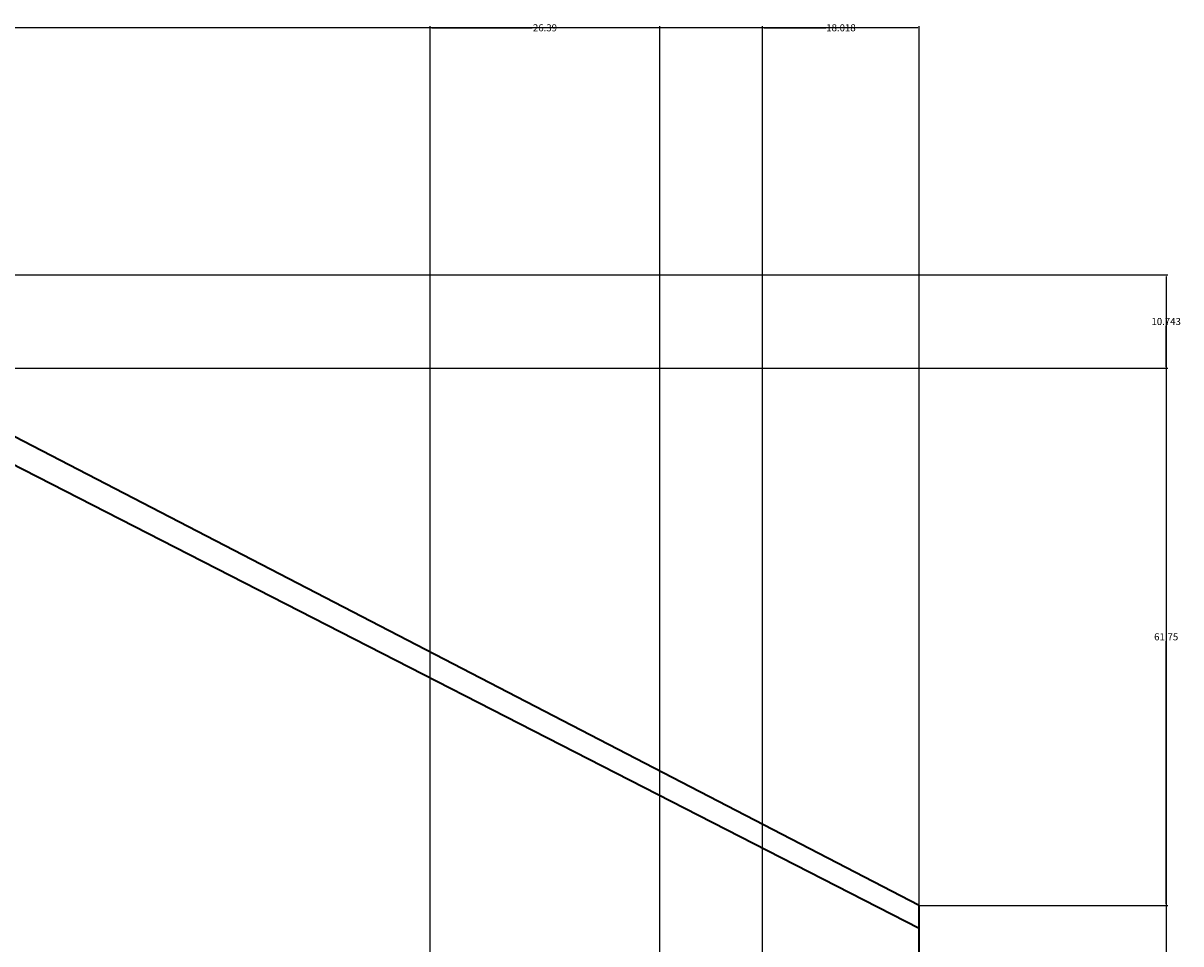
# Model space of a CAD drawing. Units: inches. Extents: x 69 to 650, y -16 to 573.
# Tile 26 of 26: x 516 to 650, y 467 to 573. Entities that reach past the tile are written whole.
import ezdxf

# ---------------------------------------------------------------- set-up
doc = ezdxf.new("R2010")
doc.units = ezdxf.units.IN
doc.header["$MEASUREMENT"] = 0
for name, color, linetype, lineweight in [('A-ANNO-DIMS', 2, 'Continuous', 18), ('A-ROOF', 7, 'Continuous', 35), ('A-WALL', 7, 'Continuous', 35)]:
    doc.layers.add(name, color=color, linetype=linetype, lineweight=lineweight)
doc.styles.get("Standard").update_dxf_attribs({"font": 'arial.ttf'})
doc.dimstyles.get("Standard").update_dxf_attribs({"dimtxt": 0.8125, "dimasz": 0.18, "dimexe": 0.18, "dimexo": 0.0625, "dimgap": 0.09, "dimtad": 0, "dimtih": 1, "dimtoh": 1, "dimdec": 4, "dimzin": 0, "dimdsep": 46, "dimlunit": 4, "dimtxsty": 'Standard', "dimcen": 0.09, "dimadec": 0, "dimazin": 0, "dimtfac": 1, "dimtdec": 4, "dimtofl": 0, "dimtmove": 0, "dimatfit": 3, "dimfxl": 1, "dimtolj": 1, "dimtzin": 0, "dimarcsym": 0})

# ---------------------------------------------------------------- blocks, each defined once
blk = doc.blocks.new('*D19')
at = {"layer": 'A-ANNO-DIMS', "color": 0, "lineweight": -2, "transparency": 16777216}
for p, q in [((99.56, 471.72), (99.56, 572.74)), ((619.56, 87.99), (619.56, 572.74)), ((99.74, 572.56), (358.57, 572.56)), ((619.38, 572.56), (360.54, 572.56))]:
    blk.add_line(p, q, dxfattribs=at)
at = {"layer": 'A-ANNO-DIMS', "color": 0, "transparency": 16777216}
for points in [[(99.74, 572.59), (99.74, 572.53), (99.56, 572.56)], [(619.38, 572.59), (619.38, 572.53), (619.56, 572.56)]]:
    blk.add_solid(points, dxfattribs=at)
at = {"layer": 'Defpoints', "color": 0, "transparency": 16777216}
for p in [(619.56, 572.56), (99.56, 471.66), (619.56, 87.93)]:
    blk.add_point(p, dxfattribs=at)
at = {"layer": 'A-ANNO-DIMS', "color": 0, "transparency": 16777216, "insert": (359.56, 572.56), "char_height": 0.812, "attachment_point": 5}
blk.add_mtext('\\A1;520', dxfattribs=at)
blk = doc.blocks.new('*D20')
at = {"layer": 'A-ANNO-DIMS', "color": 0, "lineweight": -2, "transparency": 16777216}
for p, q in [((504.24, 544.16), (648.14, 544.16)), ((647.96, 543.98), (647.96, 304.55)), ((647.96, 64.11), (647.96, 303.54)), ((619.62, 63.93), (648.14, 63.93))]:
    blk.add_line(p, q, dxfattribs=at)
at = {"layer": 'A-ANNO-DIMS', "color": 0, "transparency": 16777216}
for points in [[(647.93, 543.98), (647.99, 543.98), (647.96, 544.16)], [(647.93, 64.11), (647.99, 64.11), (647.96, 63.93)]]:
    blk.add_solid(points, dxfattribs=at)
at = {"layer": 'Defpoints', "color": 0, "transparency": 16777216}
for p in [(504.18, 544.16), (647.96, 544.16), (619.56, 63.93)]:
    blk.add_point(p, dxfattribs=at)
at = {"layer": 'A-ANNO-DIMS', "color": 0, "transparency": 16777216, "insert": (647.96, 304.04), "char_height": 0.812, "attachment_point": 5}
blk.add_mtext('\\A1;480.2', dxfattribs=at)
blk = doc.blocks.new('*D48')
at = {"layer": 'A-ANNO-DIMS', "color": 0, "lineweight": -2, "transparency": 16777216}
for p, q in [((619.62, 471.66), (648.14, 471.66)), ((647.96, 471.48), (647.96, 442.3)), ((647.96, 412.11), (647.96, 441.29)), ((619.62, 411.93), (648.14, 411.93))]:
    blk.add_line(p, q, dxfattribs=at)
at = {"layer": 'A-ANNO-DIMS', "color": 0, "transparency": 16777216}
for points in [[(647.93, 471.48), (647.99, 471.48), (647.96, 471.66)], [(647.93, 412.11), (647.99, 412.11), (647.96, 411.93)]]:
    blk.add_solid(points, dxfattribs=at)
at = {"layer": 'Defpoints', "color": 0, "transparency": 16777216}
for p in [(619.56, 471.66), (647.96, 471.66), (619.56, 411.93)]:
    blk.add_point(p, dxfattribs=at)
at = {"layer": 'A-ANNO-DIMS', "color": 0, "transparency": 16777216, "insert": (647.96, 441.79), "char_height": 0.812, "attachment_point": 5}
blk.add_mtext('\\A1;59.73', dxfattribs=at)
blk = doc.blocks.new('*D51')
at = {"layer": 'A-ANNO-DIMS', "color": 0, "lineweight": -2, "transparency": 16777216}
for p, q in [((500.33, 533.41), (648.14, 533.41)), ((647.96, 533.23), (647.96, 503.04)), ((647.96, 471.84), (647.96, 502.03)), ((619.62, 471.66), (648.14, 471.66))]:
    blk.add_line(p, q, dxfattribs=at)
at = {"layer": 'A-ANNO-DIMS', "color": 0, "transparency": 16777216}
for points in [[(647.93, 533.23), (647.99, 533.23), (647.96, 533.41)], [(647.93, 471.84), (647.99, 471.84), (647.96, 471.66)]]:
    blk.add_solid(points, dxfattribs=at)
at = {"layer": 'Defpoints', "color": 0, "transparency": 16777216}
for p in [(500.26, 533.41), (647.96, 533.41), (619.56, 471.66)]:
    blk.add_point(p, dxfattribs=at)
at = {"layer": 'A-ANNO-DIMS', "color": 0, "transparency": 16777216, "insert": (647.96, 502.54), "char_height": 0.812, "attachment_point": 5}
blk.add_mtext('\\A1;61.75', dxfattribs=at)
blk = doc.blocks.new('*D52')
at = {"layer": 'A-ANNO-DIMS', "color": 0, "lineweight": -2, "transparency": 16777216}
for p, q in [((504.24, 544.16), (648.14, 544.16)), ((647.96, 543.98), (647.96, 539.29)), ((647.96, 533.59), (647.96, 538.28)), ((500.33, 533.41), (648.14, 533.41))]:
    blk.add_line(p, q, dxfattribs=at)
at = {"layer": 'A-ANNO-DIMS', "color": 0, "transparency": 16777216}
for points in [[(647.93, 543.98), (647.99, 543.98), (647.96, 544.16)], [(647.93, 533.59), (647.99, 533.59), (647.96, 533.41)]]:
    blk.add_solid(points, dxfattribs=at)
at = {"layer": 'Defpoints', "color": 0, "transparency": 16777216}
for p in [(504.18, 544.16), (647.96, 544.16), (500.26, 533.41)]:
    blk.add_point(p, dxfattribs=at)
at = {"layer": 'A-ANNO-DIMS', "color": 0, "transparency": 16777216, "insert": (647.96, 538.79), "char_height": 0.812, "attachment_point": 5}
blk.add_mtext('\\A1;10.743', dxfattribs=at)
blk = doc.blocks.new('*D55')
at = {"layer": 'A-ANNO-DIMS', "color": 0, "lineweight": -2, "transparency": 16777216}
for p, q in [((563.31, 414.48), (563.31, 572.74)), ((589.7, 414.48), (589.7, 572.74)), ((563.49, 572.56), (575.03, 572.56)), ((589.52, 572.56), (577.97, 572.56))]:
    blk.add_line(p, q, dxfattribs=at)
at = {"layer": 'A-ANNO-DIMS', "color": 0, "transparency": 16777216}
for points in [[(563.49, 572.59), (563.49, 572.53), (563.31, 572.56)], [(589.52, 572.59), (589.52, 572.53), (589.7, 572.56)]]:
    blk.add_solid(points, dxfattribs=at)
at = {"layer": 'Defpoints', "color": 0, "transparency": 16777216}
for p in [(589.7, 572.56), (563.31, 414.41), (589.7, 414.41)]:
    blk.add_point(p, dxfattribs=at)
at = {"layer": 'A-ANNO-DIMS', "color": 0, "transparency": 16777216, "insert": (576.5, 572.56), "char_height": 0.812, "attachment_point": 5}
blk.add_mtext('\\A1;26.39', dxfattribs=at)
blk = doc.blocks.new('*D56')
at = {"layer": 'A-ANNO-DIMS', "color": 0, "lineweight": -2, "transparency": 16777216}
for p, q in [((601.54, 414.48), (601.54, 572.74)), ((619.56, 411.99), (619.56, 572.74)), ((601.72, 572.56), (608.81, 572.56)), ((619.38, 572.56), (612.29, 572.56))]:
    blk.add_line(p, q, dxfattribs=at)
at = {"layer": 'A-ANNO-DIMS', "color": 0, "transparency": 16777216}
for points in [[(601.72, 572.59), (601.72, 572.53), (601.54, 572.56)], [(619.38, 572.59), (619.38, 572.53), (619.56, 572.56)]]:
    blk.add_solid(points, dxfattribs=at)
at = {"layer": 'Defpoints', "color": 0, "transparency": 16777216}
for p in [(619.56, 572.56), (601.54, 414.41), (619.56, 411.93)]:
    blk.add_point(p, dxfattribs=at)
at = {"layer": 'A-ANNO-DIMS', "color": 0, "transparency": 16777216, "insert": (610.55, 572.56), "char_height": 0.812, "attachment_point": 5}
blk.add_mtext('\\A1;18.018', dxfattribs=at)

msp = doc.modelspace()

# ---------------------------------------------------------------- linework, layer by layer
at = {"layer": 'A-ROOF'}
for p, q in [((619.555, 471.6595), (500.263, 533.4142)), ((619.555, 468.9953), (500.263, 530.0442))]:
    msp.add_line(p, q, dxfattribs=at)
at = {"layer": 'A-WALL'}
msp.add_line((619.555, 411.93), (619.555, 471.6595), dxfattribs=at)

# ---------------------------------------------------------------- dimensions: what is measured, and where the dimension line sits
at = {"layer": 'A-ANNO-DIMS'}
for base, p1, p2, override, picture, middle in [((619.555, 572.5573), (99.556, 471.6595), (619.555, 87.93), {"dimdec": 0, "dimlfac": 1, "dimrnd": 0, "dimzin": 0, "dimdsep": 46, "dimlunit": 2}, '*D19', (359.5555, 572.5573)), ((589.6958, 572.5573), (563.3054, 414.4146), (589.6958, 414.4146), {"dimdec": 2, "dimlfac": 1, "dimrnd": 0, "dimzin": 0, "dimdsep": 46, "dimlunit": 2}, '*D55', (576.5006, 572.5573)), ((619.555, 572.5573), (601.5371, 414.4146), (619.555, 411.93), {"dimdec": 3, "dimlfac": 1, "dimrnd": 0, "dimzin": 0, "dimdsep": 46, "dimlunit": 2}, '*D56', (610.5461, 572.5573))]:
    dim = msp.add_linear_dim(base=base, p1=p1, p2=p2, dimstyle='Standard', override=override, dxfattribs=at)
    dim.commit()
    dim.dimension.update_dxf_attribs({"geometry": picture, "text_midpoint": middle})
for base, p1, p2, override, picture, middle in [((647.955, 544.1573), (500.263, 533.4142), (504.1763, 544.1573), {"dimdec": 3, "dimlfac": 1, "dimrnd": 0, "dimzin": 0, "dimdsep": 46, "dimlunit": 2}, '*D52', (647.955, 538.7857)), ((647.955, 544.1573), (619.555, 63.93), (504.1763, 544.1573), {"dimdec": 1, "dimlfac": 1, "dimrnd": 0, "dimzin": 0, "dimdsep": 46, "dimlunit": 2}, '*D20', (647.955, 304.0436)), ((647.955, 533.4142), (619.555, 471.6595), (500.263, 533.4142), {"dimdec": 2, "dimlfac": 1, "dimrnd": 0, "dimzin": 0, "dimdsep": 46, "dimlunit": 2}, '*D51', (647.955, 502.5368)), ((647.955, 471.6595), (619.555, 411.93), (619.555, 471.6595), {"dimdec": 2, "dimlfac": 1, "dimrnd": 0, "dimzin": 0, "dimdsep": 46, "dimlunit": 2}, '*D48', (647.955, 441.7948))]:
    dim = msp.add_linear_dim(base=base, p1=p1, p2=p2, angle=90, dimstyle='Standard', override=override, dxfattribs=at)
    dim.commit()
    dim.dimension.update_dxf_attribs({"geometry": picture, "text_midpoint": middle})

doc.saveas('drawing.dxf')
